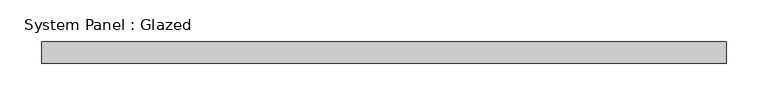
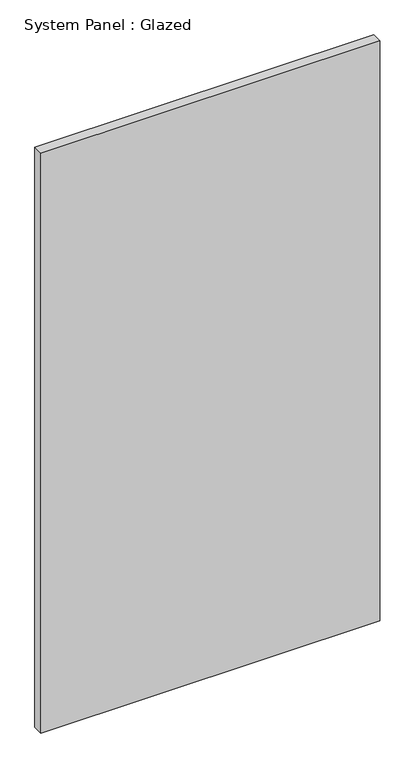
"""IFC4 building model written with IfcOpenShell, lengths in millimetres: plate geometry, System Panel : Glazed."""

from ifc_helpers import new_model, si_unit, origin, origin_with_axes, place, context, project, spatial, polyline, outline, extrude, source, transform, mapped, element, save


def system_panel_glazed_abee1f72(model_context):
    return source(origin(), model_context, "Body", "SweptSolid", [
        extrude(outline(polyline([(409.575, 19.05), (-409.575, 19.05), (-409.575, 44.45), (409.575, 44.45), (409.575, 19.05)])), origin_with_axes(), (0.0, 0.0, 1.0), 1483.0660092),
    ])


if __name__ == "__main__":
    model = new_model("IFC4")
    model_context = context("Model", 3, world=origin())
    ifc_project = project(units=[si_unit("LENGTHUNIT", "METRE", prefix="MILLI")], contexts=[model_context])
    site = spatial("IfcSite", under=ifc_project)
    building = spatial("IfcBuilding", under=site)
    placement = place(None, origin())
    system_panel_glazed_shape = system_panel_glazed_abee1f72(model_context)
    element("IfcPlate", 1, ObjectType="System Panel : Glazed", at=placement, inside=building, context=model_context, shape_type="MappedRepresentation", body=[
        mapped(system_panel_glazed_shape, transform((0.0, 0.0, 0.0), x_axis=(1.0, 0.0, 0.0), y_axis=(0.0, 1.0, 0.0), z_axis=(0.0, 0.0, 1.0))),
    ])
    save(model, "model.ifc")

# Revit data of these elements
# Type "System Panel : Glazed"
#   Construction Type Id = "GSP4R"
#   Analytic Construction = "1/8 in Pilkington single glazing"
#   Visual Light Transmittance = 0.9
#   Solar Heat Gain Coefficient = 0.86
#   Heat Transfer Coefficient (U) = 1.18115 BTU/(h·ft²·°F)
#   Define Thermal Properties by = 1
# Element 1 (IfcPlate, "System Panel : Glazed")
#   Materials on its faces: "Glass"
# Materials
#   "Glass": class "Glass", colour RGB 0 128 192, transparency 0.75, Description = "Soda Lime Glass", Cost = 0
